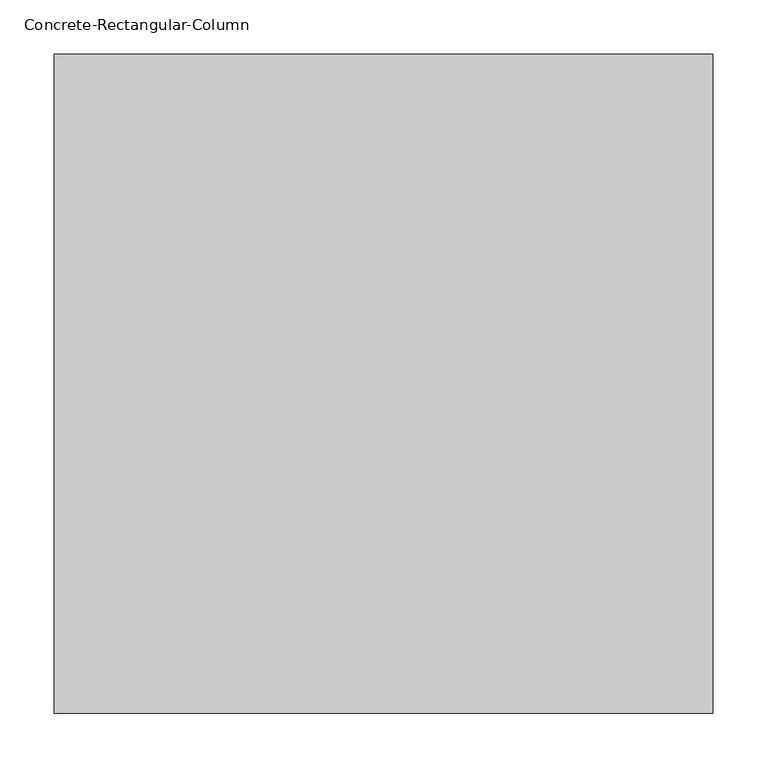
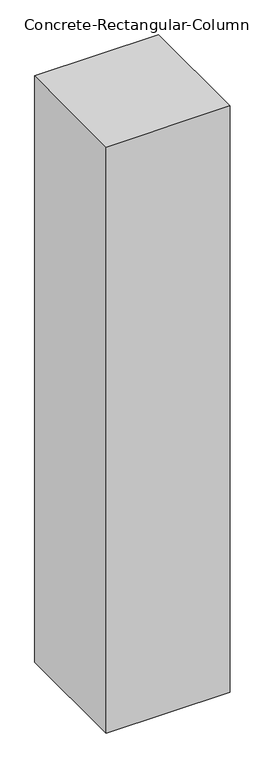
"""IFC4 building model written with IfcOpenShell, lengths in millimetres: column geometry, Concrete-Rectangular-Column."""

from ifc_helpers import new_model, si_unit, origin, origin_with_axes, place, context, project, spatial, polyline, outline, extrude, source, transform, mapped, element, save


def concrete_rectangular_column_c091e905(model_context):
    return source(origin(), model_context, "Body", "SweptSolid", [
        extrude(outline(polyline([(304.8, 304.8), (304.8, -304.8), (-304.8, -304.8), (-304.8, 304.8), (304.8, 304.8)])), origin_with_axes(), (0.0, 0.0, 1.0), 3048.0),
    ])


if __name__ == "__main__":
    model = new_model("IFC4")
    model_context = context("Model", 3, world=origin())
    ifc_project = project(units=[si_unit("LENGTHUNIT", "METRE", prefix="MILLI")], contexts=[model_context])
    site = spatial("IfcSite", under=ifc_project)
    building = spatial("IfcBuilding", under=site)
    placement = place(None, origin())
    concrete_rectangular_column_shape = concrete_rectangular_column_c091e905(model_context)
    element("IfcColumn", 1, ObjectType="Concrete-Rectangular-Column", at=placement, inside=building, context=model_context, shape_type="MappedRepresentation", body=[
        mapped(concrete_rectangular_column_shape, transform((0.0, 0.0, 0.0), x_axis=(1.0, 0.0, 0.0), y_axis=(0.0, 1.0, 0.0), z_axis=(0.0, 0.0, 1.0))),
    ])
    save(model, "model.ifc")

# Revit data of these elements
# Type "Concrete-Rectangular-Column"
#   Assembly Code = "B10"
#   b = 2' - 0"
#   h = 2' - 0"
#   Structural Material [instance default] = Concrete, Cast-in-Place gray
# Element 1 (IfcColumn, "Concrete-Rectangular-Column")
#   Structural Material = Concrete
#   Materials on its faces: "Concrete"
# Materials
#   "Concrete, Cast-in-Place gray": class "Concrete", colour RGB 192 192 192, transparency 0, Description = "Cast-in-place concrete", Cost = 0
#   "Concrete": class "Concrete", colour RGB 120 120 120, transparency 0, Description = "Portland Cement Concrete", Cost = 0
